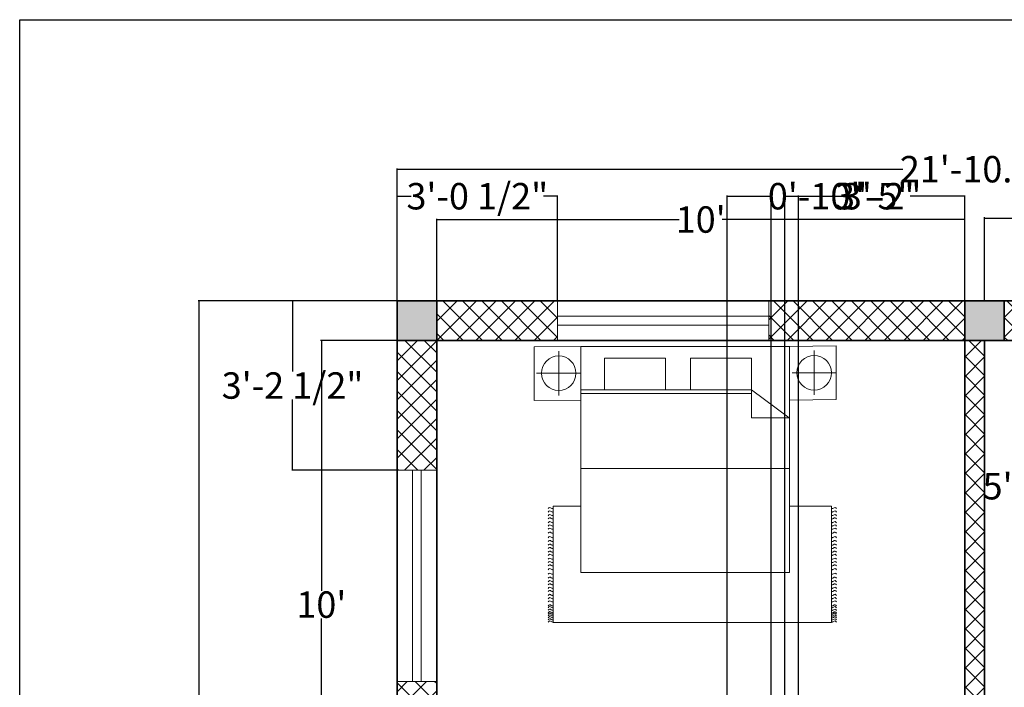
# Model space of a CAD drawing. Units: inches. Extents: x 958 to 1375, y 3152 to 3689.
# Tile 6 of 8: x 958 to 1182, y 3538 to 3689. Entities that reach past the tile are written whole.
import ezdxf

# ---------------------------------------------------------------- set-up
doc = ezdxf.new("R2010")
doc.units = ezdxf.units.IN
doc.header["$MEASUREMENT"] = 0
for name, color, linetype, lineweight in [('A-ANNO-DIMS', 2, 'Continuous', 18), ('A-ANNO-TTLB', 7, 'Continuous', 25), ('A-COLS', 7, 'Continuous', 35), ('A-FURN', 8, 'Continuous', 18), ('A-WALL', 7, 'Continuous', 35), ('windows', 140, 'Continuous', 18)]:
    doc.layers.add(name, color=color, linetype=linetype, lineweight=lineweight)
doc.layers.add('A-COLS-PATT', color=18, linetype='Continuous', lineweight=13, true_color=0x000000)
doc.layers.add('A-WALL-PATT', color=240, linetype='Continuous', lineweight=13, true_color=0xed1f24)
doc.styles.get("Standard").update_dxf_attribs({"font": 'arial.ttf'})
doc.dimstyles.get("Standard").update_dxf_attribs({"dimtxt": 6, "dimasz": 0.18, "dimexe": 0.18, "dimexo": 0.0625, "dimgap": 0.09, "dimtad": 0, "dimtih": 1, "dimtoh": 1, "dimdec": 1, "dimzin": 0, "dimdsep": 46, "dimlunit": 3, "dimtxsty": 'Standard', "dimcen": 0.09, "dimadec": 0, "dimazin": 0, "dimtfac": 1, "dimtdec": 1, "dimtofl": 0, "dimtmove": 0, "dimatfit": 3, "dimfxl": 1, "dimtolj": 1, "dimtzin": 0, "dimarcsym": 0})

# ---------------------------------------------------------------- blocks, each defined once
blk = doc.blocks.new('*D3')
at = {"layer": 'A-ANNO-DIMS', "color": 0, "lineweight": -2, "transparency": 16777216}
for p, q in [((1053.2, 3625.6), (1053.2, 3644.17)), ((1053.38, 3643.99), (1108.3, 3643.99)), ((1173.02, 3643.99), (1118.1, 3643.99)), ((1173.2, 3625.6), (1173.2, 3644.17))]:
    blk.add_line(p, q, dxfattribs=at)
at = {"layer": 'A-ANNO-DIMS', "color": 0, "transparency": 16777216}
for points in [[(1053.38, 3644.02), (1053.38, 3643.96), (1053.2, 3643.99)], [(1173.02, 3644.02), (1173.02, 3643.96), (1173.2, 3643.99)]]:
    blk.add_solid(points, dxfattribs=at)
at = {"layer": 'Defpoints', "color": 0, "transparency": 16777216}
for p in [(1173.2, 3643.99), (1053.2, 3625.53), (1173.2, 3625.53)]:
    blk.add_point(p, dxfattribs=at)
at = {"layer": 'A-ANNO-DIMS', "color": 0, "transparency": 16777216, "insert": (1113.2, 3643.99), "char_height": 6, "attachment_point": 5}
blk.add_mtext("\\A1;10'", dxfattribs=at)
blk = doc.blocks.new('*D4')
at = {"layer": 'A-ANNO-DIMS', "color": 0, "lineweight": -2, "transparency": 16777216}
for p, q in [((1177.7, 3625.6), (1177.7, 3644.49)), ((1177.88, 3644.31), (1232.8, 3644.31)), ((1297.52, 3644.31), (1242.6, 3644.31)), ((1297.7, 3625.6), (1297.7, 3644.49))]:
    blk.add_line(p, q, dxfattribs=at)
at = {"layer": 'A-ANNO-DIMS', "color": 0, "transparency": 16777216}
for points in [[(1177.88, 3644.34), (1177.88, 3644.28), (1177.7, 3644.31)], [(1297.52, 3644.34), (1297.52, 3644.28), (1297.7, 3644.31)]]:
    blk.add_solid(points, dxfattribs=at)
at = {"layer": 'Defpoints', "color": 0, "transparency": 16777216}
for p in [(1297.7, 3644.31), (1177.7, 3625.53), (1297.7, 3625.53)]:
    blk.add_point(p, dxfattribs=at)
at = {"layer": 'A-ANNO-DIMS', "color": 0, "transparency": 16777216, "insert": (1237.7, 3644.31), "char_height": 6, "attachment_point": 5}
blk.add_mtext("\\A1;10'", dxfattribs=at)
blk = doc.blocks.new('*D11')
at = {"layer": 'A-ANNO-DIMS', "color": 0, "lineweight": -2, "transparency": 16777216}
for p, q in [((1044.2, 3625.6), (1044.2, 3655.6)), ((1044.38, 3655.42), (1159.17, 3655.42)), ((1306.52, 3655.42), (1191.72, 3655.42)), ((1306.7, 3625.6), (1306.7, 3655.6))]:
    blk.add_line(p, q, dxfattribs=at)
at = {"layer": 'A-ANNO-DIMS', "color": 0, "transparency": 16777216}
for points in [[(1044.38, 3655.45), (1044.38, 3655.39), (1044.2, 3655.42)], [(1306.52, 3655.45), (1306.52, 3655.39), (1306.7, 3655.42)]]:
    blk.add_solid(points, dxfattribs=at)
at = {"layer": 'Defpoints', "color": 0, "transparency": 16777216}
for p in [(1306.7, 3655.42), (1044.2, 3625.53), (1306.7, 3625.53)]:
    blk.add_point(p, dxfattribs=at)
at = {"layer": 'A-ANNO-DIMS', "color": 0, "transparency": 16777216, "insert": (1175.45, 3655.42), "char_height": 6, "attachment_point": 5}
blk.add_mtext('\\A1;21\'-10.5"', dxfattribs=at)
blk = doc.blocks.new('*D12')
at = {"layer": 'A-ANNO-DIMS', "color": 0, "lineweight": -2, "transparency": 16777216}
for p, q in [((1044.13, 3616.53), (1026.81, 3616.53)), ((1026.99, 3616.35), (1026.99, 3559.69)), ((1026.99, 3496.71), (1026.99, 3553.38)), ((1044.13, 3496.53), (1026.81, 3496.53))]:
    blk.add_line(p, q, dxfattribs=at)
at = {"layer": 'A-ANNO-DIMS', "color": 0, "transparency": 16777216}
for points in [[(1026.96, 3616.35), (1027.02, 3616.35), (1026.99, 3616.53)], [(1026.96, 3496.71), (1027.02, 3496.71), (1026.99, 3496.53)]]:
    blk.add_solid(points, dxfattribs=at)
at = {"layer": 'Defpoints', "color": 0, "transparency": 16777216}
for p in [(1044.2, 3616.53), (1026.99, 3496.53), (1044.2, 3496.53)]:
    blk.add_point(p, dxfattribs=at)
at = {"layer": 'A-ANNO-DIMS', "color": 0, "transparency": 16777216, "insert": (1026.99, 3556.53), "char_height": 6, "attachment_point": 5}
blk.add_mtext("\\A1;10'", dxfattribs=at)
blk = doc.blocks.new('*D15')
at = {"layer": 'A-ANNO-DIMS', "color": 0, "lineweight": -2, "transparency": 16777216}
for p, q in [((1044.13, 3625.53), (998.97, 3625.53)), ((999.15, 3625.35), (999.15, 3444.94)), ((999.15, 3258.21), (999.15, 3438.63)), ((1044.13, 3258.03), (998.97, 3258.03))]:
    blk.add_line(p, q, dxfattribs=at)
at = {"layer": 'A-ANNO-DIMS', "color": 0, "transparency": 16777216}
for points in [[(999.12, 3625.35), (999.18, 3625.35), (999.15, 3625.53)], [(999.12, 3258.21), (999.18, 3258.21), (999.15, 3258.03)]]:
    blk.add_solid(points, dxfattribs=at)
at = {"layer": 'Defpoints', "color": 0, "transparency": 16777216}
for p in [(1044.2, 3625.53), (999.15, 3258.03), (1044.2, 3258.03)]:
    blk.add_point(p, dxfattribs=at)
at = {"layer": 'A-ANNO-DIMS', "color": 0, "transparency": 16777216, "insert": (999.15, 3441.78), "char_height": 6, "attachment_point": 5}
blk.add_mtext('\\A1;30\'-7.5"', dxfattribs=at)
blk = doc.blocks.new('BED-DOUBLE')
for p, q in [((5.6, 61.62), (5.6, 51.56)), ((63.65, 61.72), (63.65, 51.66)), ((10.63, 56.59), (0.57, 56.59)), ((68.68, 56.69), (58.62, 56.69)), ((49.39, 52.82), (10.63, 52.82)), ((49.44, 52), (10.63, 52)), ((49.39, 52.82), (58, 46.47)), ((49.44, 52.82), (49.44, 46.47)), ((49.44, 46.47), (58, 46.47)), ((58.05, 34.96), (10.63, 34.96)), ((4.36, 0), (4.36, 26.37)), ((4.36, 26.37), (10.65, 26.37)), ((58.05, 26.37), (67.59, 26.37)), ((67.59, 26.37), (67.59, 0)), ((67.59, 0), (4.36, 0))]:
    blk.add_line(p, q)
for points in [[(0, 50.39), (10.63, 50.5), (10.63, 62.68), (0, 62.58)], [(58.05, 62.68), (58.05, 11.37), (10.63, 11.37), (10.63, 62.68)], [(58.05, 50.5), (68.68, 50.6), (68.68, 62.78), (58.05, 62.68)], [(29.88, 59.98), (29.88, 52.82), (15.98, 52.82), (15.98, 59.98)], [(49.44, 59.98), (49.44, 52.82), (35.55, 52.82), (35.55, 59.98)]]:
    blk.add_lwpolyline(points, close=True)
for centre in [(5.6, 56.59), (63.65, 56.69)]:
    blk.add_circle(centre, 3.92)
for points, knots in [([(3.23, 25.84), (3.32, 25.96), (3.52, 26.2), (3.86, 25.96), (4.14, 25.78), (4.29, 25.89), (4.36, 25.94)], [0, 0, 0, 0, 0.400747, 0.791423, 1.067667, 1.29709, 1.29709, 1.29709, 1.29709]), ([(3.23, 25.06), (3.32, 25.18), (3.52, 25.42), (3.86, 25.18), (4.14, 25.01), (4.29, 25.11), (4.36, 25.16)], [0, 0, 0, 0, 0.400747, 0.791423, 1.067667, 1.29709, 1.29709, 1.29709, 1.29709]), ([(68.71, 25.84), (68.61, 25.96), (68.42, 26.2), (68.08, 25.96), (67.8, 25.78), (67.65, 25.89), (67.58, 25.94)], [0, 0, 0, 0, 0.400747, 0.791423, 1.067667, 1.29709, 1.29709, 1.29709, 1.29709]), ([(68.71, 25.06), (68.61, 25.18), (68.42, 25.42), (68.08, 25.18), (67.8, 25.01), (67.65, 25.11), (67.58, 25.16)], [0, 0, 0, 0, 0.400747, 0.791423, 1.067667, 1.29709, 1.29709, 1.29709, 1.29709]), ([(3.23, 24.24), (3.32, 24.36), (3.52, 24.6), (3.86, 24.36), (4.14, 24.19), (4.29, 24.3), (4.36, 24.34)], [0, 0, 0, 0, 0.400747, 0.791423, 1.067667, 1.29709, 1.29709, 1.29709, 1.29709]), ([(3.23, 23.51), (3.32, 23.63), (3.52, 23.87), (3.86, 23.63), (4.14, 23.46), (4.29, 23.57), (4.36, 23.62)], [0, 0, 0, 0, 0.400747, 0.791423, 1.067667, 1.29709, 1.29709, 1.29709, 1.29709]), ([(3.23, 22.63), (3.32, 22.75), (3.52, 22.99), (3.86, 22.75), (4.14, 22.58), (4.29, 22.69), (4.36, 22.73)], [0, 0, 0, 0, 0.400747, 0.791423, 1.067667, 1.29709, 1.29709, 1.29709, 1.29709]), ([(68.71, 24.24), (68.61, 24.36), (68.42, 24.6), (68.08, 24.36), (67.8, 24.19), (67.65, 24.3), (67.58, 24.34)], [0, 0, 0, 0, 0.400747, 0.791423, 1.067667, 1.29709, 1.29709, 1.29709, 1.29709]), ([(68.71, 23.51), (68.61, 23.63), (68.42, 23.87), (68.08, 23.63), (67.8, 23.46), (67.65, 23.57), (67.58, 23.62)], [0, 0, 0, 0, 0.400747, 0.791423, 1.067667, 1.29709, 1.29709, 1.29709, 1.29709]), ([(68.71, 22.63), (68.61, 22.75), (68.42, 22.99), (68.08, 22.75), (67.8, 22.58), (67.65, 22.69), (67.58, 22.73)], [0, 0, 0, 0, 0.400747, 0.791423, 1.067667, 1.29709, 1.29709, 1.29709, 1.29709]), ([(3.23, 21.88), (3.32, 22), (3.52, 22.24), (3.86, 22), (4.14, 21.83), (4.29, 21.93), (4.36, 21.98)], [0, 0, 0, 0, 0.400747, 0.791423, 1.067667, 1.29709, 1.29709, 1.29709, 1.29709]), ([(3.23, 21.15), (3.32, 21.27), (3.52, 21.51), (3.86, 21.27), (4.14, 21.1), (4.29, 21.21), (4.36, 21.25)], [0, 0, 0, 0, 0.400747, 0.791423, 1.067667, 1.29709, 1.29709, 1.29709, 1.29709]), ([(3.23, 20.27), (3.32, 20.39), (3.52, 20.63), (3.86, 20.39), (4.14, 20.22), (4.29, 20.32), (4.36, 20.37)], [0, 0, 0, 0, 0.400747, 0.791423, 1.067667, 1.29709, 1.29709, 1.29709, 1.29709]), ([(68.71, 21.88), (68.61, 22), (68.42, 22.24), (68.08, 22), (67.8, 21.83), (67.65, 21.93), (67.58, 21.98)], [0, 0, 0, 0, 0.400747, 0.791423, 1.067667, 1.29709, 1.29709, 1.29709, 1.29709]), ([(68.71, 21.15), (68.61, 21.27), (68.42, 21.51), (68.08, 21.27), (67.8, 21.1), (67.65, 21.21), (67.58, 21.25)], [0, 0, 0, 0, 0.400747, 0.791423, 1.067667, 1.29709, 1.29709, 1.29709, 1.29709]), ([(68.71, 20.27), (68.61, 20.39), (68.42, 20.63), (68.08, 20.39), (67.8, 20.22), (67.65, 20.32), (67.58, 20.37)], [0, 0, 0, 0, 0.400747, 0.791423, 1.067667, 1.29709, 1.29709, 1.29709, 1.29709]), ([(3.23, 19.23), (3.32, 19.35), (3.52, 19.59), (3.86, 19.35), (4.14, 19.18), (4.29, 19.29), (4.36, 19.33)], [0, 0, 0, 0, 0.400747, 0.791423, 1.067667, 1.29709, 1.29709, 1.29709, 1.29709]), ([(3.23, 18.35), (3.32, 18.47), (3.52, 18.71), (3.86, 18.47), (4.14, 18.3), (4.29, 18.4), (4.36, 18.45)], [0, 0, 0, 0, 0.400747, 0.791423, 1.067667, 1.29709, 1.29709, 1.29709, 1.29709]), ([(68.71, 19.23), (68.61, 19.35), (68.42, 19.59), (68.08, 19.35), (67.8, 19.18), (67.65, 19.29), (67.58, 19.33)], [0, 0, 0, 0, 0.400747, 0.791423, 1.067667, 1.29709, 1.29709, 1.29709, 1.29709]), ([(68.71, 18.35), (68.61, 18.47), (68.42, 18.71), (68.08, 18.47), (67.8, 18.3), (67.65, 18.4), (67.58, 18.45)], [0, 0, 0, 0, 0.400747, 0.791423, 1.067667, 1.29709, 1.29709, 1.29709, 1.29709]), ([(3.23, 17.53), (3.32, 17.65), (3.52, 17.89), (3.86, 17.65), (4.14, 17.48), (4.29, 17.59), (4.36, 17.64)], [0, 0, 0, 0, 0.400747, 0.791423, 1.067667, 1.29709, 1.29709, 1.29709, 1.29709]), ([(3.23, 16.76), (3.32, 16.88), (3.52, 17.12), (3.86, 16.88), (4.14, 16.71), (4.29, 16.81), (4.36, 16.86)], [0, 0, 0, 0, 0.400747, 0.791423, 1.067667, 1.29709, 1.29709, 1.29709, 1.29709]), ([(3.23, 15.94), (3.32, 16.06), (3.52, 16.3), (3.86, 16.06), (4.14, 15.89), (4.29, 16), (4.36, 16.04)], [0, 0, 0, 0, 0.400747, 0.791423, 1.067667, 1.29709, 1.29709, 1.29709, 1.29709]), ([(68.71, 17.53), (68.61, 17.65), (68.42, 17.89), (68.08, 17.65), (67.8, 17.48), (67.65, 17.59), (67.58, 17.64)], [0, 0, 0, 0, 0.400747, 0.791423, 1.067667, 1.29709, 1.29709, 1.29709, 1.29709]), ([(68.71, 16.76), (68.61, 16.88), (68.42, 17.12), (68.08, 16.88), (67.8, 16.71), (67.65, 16.81), (67.58, 16.86)], [0, 0, 0, 0, 0.400747, 0.791423, 1.067667, 1.29709, 1.29709, 1.29709, 1.29709]), ([(68.71, 15.94), (68.61, 16.06), (68.42, 16.3), (68.08, 16.06), (67.8, 15.89), (67.65, 16), (67.58, 16.04)], [0, 0, 0, 0, 0.400747, 0.791423, 1.067667, 1.29709, 1.29709, 1.29709, 1.29709]), ([(3.23, 15.21), (3.32, 15.33), (3.52, 15.57), (3.86, 15.33), (4.14, 15.16), (4.29, 15.27), (4.36, 15.32)], [0, 0, 0, 0, 0.400747, 0.791423, 1.067667, 1.29709, 1.29709, 1.29709, 1.29709]), ([(3.23, 14.33), (3.32, 14.45), (3.52, 14.69), (3.86, 14.45), (4.14, 14.28), (4.29, 14.39), (4.36, 14.43)], [0, 0, 0, 0, 0.400747, 0.791423, 1.067667, 1.29709, 1.29709, 1.29709, 1.29709]), ([(3.23, 13.58), (3.32, 13.7), (3.52, 13.94), (3.86, 13.7), (4.14, 13.53), (4.29, 13.63), (4.36, 13.68)], [0, 0, 0, 0, 0.400747, 0.791423, 1.067667, 1.29709, 1.29709, 1.29709, 1.29709]), ([(68.71, 15.21), (68.61, 15.33), (68.42, 15.57), (68.08, 15.33), (67.8, 15.16), (67.65, 15.27), (67.58, 15.32)], [0, 0, 0, 0, 0.400747, 0.791423, 1.067667, 1.29709, 1.29709, 1.29709, 1.29709]), ([(68.71, 14.33), (68.61, 14.45), (68.42, 14.69), (68.08, 14.45), (67.8, 14.28), (67.65, 14.39), (67.58, 14.43)], [0, 0, 0, 0, 0.400747, 0.791423, 1.067667, 1.29709, 1.29709, 1.29709, 1.29709]), ([(68.71, 13.58), (68.61, 13.7), (68.42, 13.94), (68.08, 13.7), (67.8, 13.53), (67.65, 13.63), (67.58, 13.68)], [0, 0, 0, 0, 0.400747, 0.791423, 1.067667, 1.29709, 1.29709, 1.29709, 1.29709]), ([(3.23, 12.85), (3.32, 12.97), (3.52, 13.21), (3.86, 12.97), (4.14, 12.8), (4.29, 12.9), (4.36, 12.95)], [0, 0, 0, 0, 0.400747, 0.791423, 1.067667, 1.29709, 1.29709, 1.29709, 1.29709]), ([(3.23, 11.97), (3.32, 12.09), (3.52, 12.33), (3.86, 12.09), (4.14, 11.92), (4.29, 12.02), (4.36, 12.07)], [0, 0, 0, 0, 0.400747, 0.791423, 1.067667, 1.29709, 1.29709, 1.29709, 1.29709]), ([(3.23, 10.93), (3.32, 11.05), (3.52, 11.29), (3.86, 11.05), (4.14, 10.88), (4.29, 10.99), (4.36, 11.03)], [0, 0, 0, 0, 0.400747, 0.791423, 1.067667, 1.29709, 1.29709, 1.29709, 1.29709]), ([(68.71, 12.85), (68.61, 12.97), (68.42, 13.21), (68.08, 12.97), (67.8, 12.8), (67.65, 12.9), (67.58, 12.95)], [0, 0, 0, 0, 0.400747, 0.791423, 1.067667, 1.29709, 1.29709, 1.29709, 1.29709]), ([(68.71, 11.97), (68.61, 12.09), (68.42, 12.33), (68.08, 12.09), (67.8, 11.92), (67.65, 12.02), (67.58, 12.07)], [0, 0, 0, 0, 0.400747, 0.791423, 1.067667, 1.29709, 1.29709, 1.29709, 1.29709]), ([(68.71, 10.93), (68.61, 11.05), (68.42, 11.29), (68.08, 11.05), (67.8, 10.88), (67.65, 10.99), (67.58, 11.03)], [0, 0, 0, 0, 0.400747, 0.791423, 1.067667, 1.29709, 1.29709, 1.29709, 1.29709]), ([(3.23, 10.05), (3.32, 10.17), (3.52, 10.41), (3.86, 10.17), (4.14, 10), (4.29, 10.1), (4.36, 10.15)], [0, 0, 0, 0, 0.400747, 0.791423, 1.067667, 1.29709, 1.29709, 1.29709, 1.29709]), ([(3.23, 9.23), (3.32, 9.35), (3.52, 9.59), (3.86, 9.35), (4.14, 9.18), (4.29, 9.29), (4.36, 9.34)], [0, 0, 0, 0, 0.400747, 0.791423, 1.067667, 1.29709, 1.29709, 1.29709, 1.29709]), ([(68.71, 10.05), (68.61, 10.17), (68.42, 10.41), (68.08, 10.17), (67.8, 10), (67.65, 10.1), (67.58, 10.15)], [0, 0, 0, 0, 0.400747, 0.791423, 1.067667, 1.29709, 1.29709, 1.29709, 1.29709]), ([(68.71, 9.23), (68.61, 9.35), (68.42, 9.59), (68.08, 9.35), (67.8, 9.18), (67.65, 9.29), (67.58, 9.34)], [0, 0, 0, 0, 0.400747, 0.791423, 1.067667, 1.29709, 1.29709, 1.29709, 1.29709]), ([(3.23, 8.54), (3.32, 8.66), (3.52, 8.9), (3.86, 8.66), (4.14, 8.49), (4.29, 8.6), (4.36, 8.65)], [0, 0, 0, 0, 0.400747, 0.791423, 1.067667, 1.29709, 1.29709, 1.29709, 1.29709]), ([(3.23, 7.73), (3.32, 7.85), (3.52, 8.09), (3.86, 7.85), (4.14, 7.68), (4.29, 7.78), (4.36, 7.83)], [0, 0, 0, 0, 0.400747, 0.791423, 1.067667, 1.29709, 1.29709, 1.29709, 1.29709]), ([(3.23, 7), (3.32, 7.12), (3.52, 7.36), (3.86, 7.12), (4.14, 6.95), (4.29, 7.05), (4.36, 7.1)], [0, 0, 0, 0, 0.400747, 0.791423, 1.067667, 1.29709, 1.29709, 1.29709, 1.29709]), ([(68.71, 8.54), (68.61, 8.66), (68.42, 8.9), (68.08, 8.66), (67.8, 8.49), (67.65, 8.6), (67.58, 8.65)], [0, 0, 0, 0, 0.400747, 0.791423, 1.067667, 1.29709, 1.29709, 1.29709, 1.29709]), ([(68.71, 7.73), (68.61, 7.85), (68.42, 8.09), (68.08, 7.85), (67.8, 7.68), (67.65, 7.78), (67.58, 7.83)], [0, 0, 0, 0, 0.400747, 0.791423, 1.067667, 1.29709, 1.29709, 1.29709, 1.29709]), ([(68.71, 7), (68.61, 7.12), (68.42, 7.36), (68.08, 7.12), (67.8, 6.95), (67.65, 7.05), (67.58, 7.1)], [0, 0, 0, 0, 0.400747, 0.791423, 1.067667, 1.29709, 1.29709, 1.29709, 1.29709]), ([(3.23, 6.12), (3.32, 6.24), (3.52, 6.48), (3.86, 6.24), (4.14, 6.07), (4.29, 6.17), (4.36, 6.22)], [0, 0, 0, 0, 0.400747, 0.791423, 1.067667, 1.29709, 1.29709, 1.29709, 1.29709]), ([(3.23, 5.37), (3.32, 5.49), (3.52, 5.73), (3.86, 5.49), (4.14, 5.31), (4.29, 5.42), (4.36, 5.47)], [0, 0, 0, 0, 0.400747, 0.791423, 1.067667, 1.29709, 1.29709, 1.29709, 1.29709]), ([(3.23, 4.64), (3.32, 4.76), (3.52, 5), (3.86, 4.76), (4.14, 4.59), (4.29, 4.69), (4.36, 4.74)], [0, 0, 0, 0, 0.400747, 0.791423, 1.067667, 1.29709, 1.29709, 1.29709, 1.29709]), ([(68.71, 6.12), (68.61, 6.24), (68.42, 6.48), (68.08, 6.24), (67.8, 6.07), (67.65, 6.17), (67.58, 6.22)], [0, 0, 0, 0, 0.400747, 0.791423, 1.067667, 1.29709, 1.29709, 1.29709, 1.29709]), ([(68.71, 5.37), (68.61, 5.49), (68.42, 5.73), (68.08, 5.49), (67.8, 5.31), (67.65, 5.42), (67.58, 5.47)], [0, 0, 0, 0, 0.400747, 0.791423, 1.067667, 1.29709, 1.29709, 1.29709, 1.29709]), ([(68.71, 4.64), (68.61, 4.76), (68.42, 5), (68.08, 4.76), (67.8, 4.59), (67.66, 4.69), (67.59, 4.73)], [0, 0, 0, 0, 0.400747, 0.791423, 1.067667, 1.283686, 1.283686, 1.283686, 1.283686]), ([(3.23, 3.75), (3.32, 3.88), (3.52, 4.12), (3.86, 3.88), (4.14, 3.7), (4.29, 3.81), (4.36, 3.86)], [0, 0, 0, 0, 0.400747, 0.791423, 1.067667, 1.29709, 1.29709, 1.29709, 1.29709]), ([(3.23, 3.33), (3.32, 3.45), (3.52, 3.7), (3.86, 3.45), (4.14, 3.27), (4.29, 3.38), (4.36, 3.43)], [0, 0, 0, 0, 0.407265, 0.802015, 1.07826, 1.307683, 1.307683, 1.307683, 1.307683]), ([(3.23, 2.76), (3.32, 2.88), (3.52, 3.12), (3.86, 2.88), (4.14, 2.71), (4.29, 2.81), (4.36, 2.86)], [0, 0, 0, 0, 0.400747, 0.791423, 1.067667, 1.29709, 1.29709, 1.29709, 1.29709]), ([(3.23, 2.19), (3.32, 2.31), (3.52, 2.55), (3.86, 2.31), (4.14, 2.13), (4.29, 2.24), (4.36, 2.29)], [0, 0, 0, 0, 0.400747, 0.791423, 1.067667, 1.29709, 1.29709, 1.29709, 1.29709]), ([(68.71, 3.75), (68.61, 3.88), (68.42, 4.12), (68.08, 3.88), (67.8, 3.7), (67.66, 3.81), (67.59, 3.85)], [0, 0, 0, 0, 0.400747, 0.791423, 1.067667, 1.283686, 1.283686, 1.283686, 1.283686]), ([(68.71, 3.33), (68.61, 3.45), (68.42, 3.69), (68.08, 3.45), (67.8, 3.28), (67.66, 3.38), (67.59, 3.42)], [0, 0, 0, 0, 0.402903, 0.794912, 1.071156, 1.287177, 1.287177, 1.287177, 1.287177]), ([(68.71, 2.73), (68.61, 2.85), (68.42, 3.09), (68.08, 2.85), (67.8, 2.68), (67.66, 2.78), (67.59, 2.83)], [0, 0, 0, 0, 0.400747, 0.791423, 1.067667, 1.283686, 1.283686, 1.283686, 1.283686]), ([(68.71, 2.16), (68.61, 2.28), (68.42, 2.52), (68.08, 2.28), (67.8, 2.11), (67.66, 2.21), (67.59, 2.25)], [0, 0, 0, 0, 0.400747, 0.791423, 1.067667, 1.283686, 1.283686, 1.283686, 1.283686]), ([(3.23, 1.88), (3.32, 2), (3.52, 2.24), (3.86, 2), (4.14, 1.82), (4.29, 1.93), (4.36, 1.98)], [0, 0, 0, 0, 0.400747, 0.791423, 1.067667, 1.29709, 1.29709, 1.29709, 1.29709]), ([(3.23, 1.46), (3.32, 1.58), (3.52, 1.82), (3.86, 1.58), (4.14, 1.41), (4.29, 1.51), (4.36, 1.56)], [0, 0, 0, 0, 0.400747, 0.791423, 1.067667, 1.29709, 1.29709, 1.29709, 1.29709]), ([(3.23, 1.06), (3.32, 1.18), (3.52, 1.42), (3.86, 1.18), (4.14, 1.01), (4.29, 1.11), (4.36, 1.16)], [0, 0, 0, 0, 0.400747, 0.791423, 1.067667, 1.29709, 1.29709, 1.29709, 1.29709]), ([(3.23, 0.57), (3.32, 0.7), (3.52, 0.94), (3.86, 0.7), (4.14, 0.52), (4.29, 0.63), (4.36, 0.68)], [0, 0, 0, 0, 0.400747, 0.791423, 1.067667, 1.29709, 1.29709, 1.29709, 1.29709]), ([(3.23, 0.07), (3.32, 0.19), (3.52, 0.43), (3.86, 0.19), (4.14, 0.02), (4.29, 0.13), (4.36, 0.18)], [0, 0, 0, 0, 0.400747, 0.791423, 1.067667, 1.29709, 1.29709, 1.29709, 1.29709]), ([(68.71, 1.43), (68.61, 1.55), (68.42, 1.79), (68.08, 1.55), (67.8, 1.38), (67.65, 1.48), (67.58, 1.53)], [0, 0, 0, 0, 0.400747, 0.791423, 1.067667, 1.29709, 1.29709, 1.29709, 1.29709]), ([(68.71, 1.03), (68.61, 1.15), (68.42, 1.39), (68.08, 1.15), (67.8, 0.98), (67.65, 1.09), (67.58, 1.13)], [0, 0, 0, 0, 0.400747, 0.791423, 1.067667, 1.29709, 1.29709, 1.29709, 1.29709]), ([(68.71, 0.55), (68.61, 0.67), (68.42, 0.91), (68.08, 0.67), (67.8, 0.5), (67.65, 0.6), (67.58, 0.65)], [0, 0, 0, 0, 0.400747, 0.791423, 1.067667, 1.29709, 1.29709, 1.29709, 1.29709]), ([(68.71, 0.07), (68.61, 0.19), (68.42, 0.43), (68.08, 0.19), (67.8, 0.02), (67.65, 0.13), (67.58, 0.18)], [0, 0, 0, 0, 0.400747, 0.791423, 1.067667, 1.29709, 1.29709, 1.29709, 1.29709]), ([(68.71, 1.85), (68.61, 1.97), (68.42, 2.21), (68.08, 1.97), (67.8, 1.8), (67.66, 1.9), (67.59, 1.94)], [0, 0, 0, 0, 0.400747, 0.791423, 1.067667, 1.283686, 1.283686, 1.283686, 1.283686])]:
    blk.add_open_spline(points, degree=3, knots=knots)
blk = doc.blocks.new('WIN-48')
for p, q in [((48, 9), (0, 9)), ((48, 5.5), (0, 5.5)), ((0, 3.5), (48, 3.5)), ((0, 0), (48, 0))]:
    blk.add_line(p, q)
blk = doc.blocks.new('*D27')
at = {"layer": 'A-ANNO-DIMS', "color": 0, "lineweight": -2, "transparency": 16777216}
for p, q in [((1205.81, 3614.81), (1195.39, 3614.81)), ((1195.57, 3614.63), (1195.57, 3586.57)), ((1195.57, 3552.21), (1195.57, 3580.26)), ((1205.81, 3552.03), (1195.39, 3552.03))]:
    blk.add_line(p, q, dxfattribs=at)
at = {"layer": 'A-ANNO-DIMS', "color": 0, "transparency": 16777216}
for points in [[(1195.54, 3614.63), (1195.6, 3614.63), (1195.57, 3614.81)], [(1195.54, 3552.21), (1195.6, 3552.21), (1195.57, 3552.03)]]:
    blk.add_solid(points, dxfattribs=at)
at = {"layer": 'Defpoints', "color": 0, "transparency": 16777216}
for p in [(1195.57, 3614.81), (1205.88, 3614.81), (1205.88, 3552.03)]:
    blk.add_point(p, dxfattribs=at)
at = {"layer": 'A-ANNO-DIMS', "color": 0, "transparency": 16777216, "insert": (1195.57, 3583.42), "char_height": 6, "attachment_point": 5}
blk.add_mtext('\\A1;5\'-3" TYP.', dxfattribs=at)
blk = doc.blocks.new('*D43')
at = {"layer": 'A-ANNO-DIMS', "color": 0, "lineweight": -2, "transparency": 16777216}
for p, q in [((1119.2, 3303.1), (1119.2, 3649.46)), ((1119.38, 3649.28), (1129.02, 3649.28)), ((1129.2, 3303.1), (1129.2, 3649.46)), ((1129.2, 3649.28), (1129.38, 3649.28))]:
    blk.add_line(p, q, dxfattribs=at)
at = {"layer": 'A-ANNO-DIMS', "color": 0, "transparency": 16777216}
for points in [[(1119.38, 3649.31), (1119.38, 3649.25), (1119.2, 3649.28)], [(1129.02, 3649.31), (1129.02, 3649.25), (1129.2, 3649.28)]]:
    blk.add_solid(points, dxfattribs=at)
at = {"layer": 'Defpoints', "color": 0, "transparency": 16777216}
for p in [(1129.2, 3649.28), (1119.2, 3303.03), (1129.2, 3303.03)]:
    blk.add_point(p, dxfattribs=at)
at = {"layer": 'A-ANNO-DIMS', "color": 0, "transparency": 16777216, "insert": (1139.77, 3649.28), "char_height": 6, "attachment_point": 5}
blk.add_mtext('\\A1;0\'-10"', dxfattribs=at)
blk = doc.blocks.new('*D44')
at = {"layer": 'A-ANNO-DIMS', "color": 0, "lineweight": -2, "transparency": 16777216}
for p, q in [((1132.32, 3267.1), (1132.32, 3649.46)), ((1132.5, 3649.28), (1144.69, 3649.28)), ((1173.02, 3649.28), (1160.82, 3649.28)), ((1173.2, 3267.1), (1173.2, 3649.46))]:
    blk.add_line(p, q, dxfattribs=at)
at = {"layer": 'A-ANNO-DIMS', "color": 0, "transparency": 16777216}
for points in [[(1132.5, 3649.31), (1132.5, 3649.25), (1132.32, 3649.28)], [(1173.02, 3649.31), (1173.02, 3649.25), (1173.2, 3649.28)]]:
    blk.add_solid(points, dxfattribs=at)
at = {"layer": 'Defpoints', "color": 0, "transparency": 16777216}
for p in [(1173.2, 3649.28), (1132.32, 3267.03), (1173.2, 3267.03)]:
    blk.add_point(p, dxfattribs=at)
at = {"layer": 'A-ANNO-DIMS', "color": 0, "transparency": 16777216, "insert": (1152.76, 3649.28), "char_height": 6, "attachment_point": 5}
blk.add_mtext('\\A1;3\'-5"', dxfattribs=at)
blk = doc.blocks.new('*D46')
at = {"layer": 'A-ANNO-DIMS', "color": 0, "lineweight": -2, "transparency": 16777216}
for p, q in [((1135.44, 3496.6), (1135.44, 3649.46)), ((1135.62, 3649.28), (1146.25, 3649.28)), ((1173.02, 3649.28), (1162.38, 3649.28)), ((1173.2, 3492.1), (1173.2, 3649.46))]:
    blk.add_line(p, q, dxfattribs=at)
at = {"layer": 'A-ANNO-DIMS', "color": 0, "transparency": 16777216}
for points in [[(1135.62, 3649.31), (1135.62, 3649.25), (1135.44, 3649.28)], [(1173.02, 3649.31), (1173.02, 3649.25), (1173.2, 3649.28)]]:
    blk.add_solid(points, dxfattribs=at)
at = {"layer": 'Defpoints', "color": 0, "transparency": 16777216}
for p in [(1173.2, 3649.28), (1135.44, 3496.53), (1173.2, 3492.03)]:
    blk.add_point(p, dxfattribs=at)
at = {"layer": 'A-ANNO-DIMS', "color": 0, "transparency": 16777216, "insert": (1154.32, 3649.28), "char_height": 6, "attachment_point": 5}
blk.add_mtext('\\A1;3\'-2"', dxfattribs=at)
blk = doc.blocks.new('*D50')
at = {"layer": 'A-ANNO-DIMS', "color": 0, "lineweight": -2, "transparency": 16777216}
for p, q in [((1044.2, 3625.6), (1044.2, 3649.46)), ((1044.38, 3649.28), (1047.39, 3649.28)), ((1080.5, 3649.28), (1077.49, 3649.28)), ((1080.68, 3625.6), (1080.68, 3649.46))]:
    blk.add_line(p, q, dxfattribs=at)
at = {"layer": 'A-ANNO-DIMS', "color": 0, "transparency": 16777216}
for points in [[(1044.38, 3649.31), (1044.38, 3649.25), (1044.2, 3649.28)], [(1080.5, 3649.31), (1080.5, 3649.25), (1080.68, 3649.28)]]:
    blk.add_solid(points, dxfattribs=at)
at = {"layer": 'Defpoints', "color": 0, "transparency": 16777216}
for p in [(1080.68, 3649.28), (1044.2, 3625.53), (1080.68, 3625.53)]:
    blk.add_point(p, dxfattribs=at)
at = {"layer": 'A-ANNO-DIMS', "color": 0, "transparency": 16777216, "insert": (1062.44, 3649.28), "char_height": 6, "attachment_point": 5}
blk.add_mtext('\\A1;3\'-0 1/2"', dxfattribs=at)
blk = doc.blocks.new('*D52')
at = {"layer": 'A-ANNO-DIMS', "color": 0, "lineweight": -2, "transparency": 16777216}
for p, q in [((1044.13, 3625.53), (1020.27, 3625.53)), ((1020.45, 3625.35), (1020.45, 3609.49)), ((1020.45, 3587.23), (1020.45, 3603.1)), ((1044.13, 3587.05), (1020.27, 3587.05))]:
    blk.add_line(p, q, dxfattribs=at)
at = {"layer": 'A-ANNO-DIMS', "color": 0, "transparency": 16777216}
for points in [[(1020.42, 3625.35), (1020.48, 3625.35), (1020.45, 3625.53)], [(1020.42, 3587.23), (1020.48, 3587.23), (1020.45, 3587.05)]]:
    blk.add_solid(points, dxfattribs=at)
at = {"layer": 'Defpoints', "color": 0, "transparency": 16777216}
for p in [(1020.45, 3625.53), (1044.2, 3625.53), (1044.2, 3587.05)]:
    blk.add_point(p, dxfattribs=at)
at = {"layer": 'A-ANNO-DIMS', "color": 0, "transparency": 16777216, "insert": (1020.45, 3606.29), "char_height": 6, "attachment_point": 5}
blk.add_mtext('\\A1;3\'-2 1/2"', dxfattribs=at)

msp = doc.modelspace()

# ---------------------------------------------------------------- hatches: boundary and pattern name
at = {"layer": 'A-COLS-PATT'}
h = msp.add_hatch(color=256, dxfattribs=at)
h.dxf.hatch_style = 1
h.paths.add_polyline_path([(1053.2, 3625.53), (1044.2, 3625.53), (1044.2, 3616.53), (1053.2, 3616.53)])
h.paths.add_polyline_path([(1182.2, 3625.53), (1173.2, 3625.53), (1173.2, 3616.53), (1182.2, 3616.53)])
h.paths.add_polyline_path([(1306.7, 3625.53), (1297.7, 3625.53), (1297.7, 3616.53), (1306.7, 3616.53)])
h.paths.add_polyline_path([(1306.7, 3501.03), (1297.7, 3501.03), (1297.7, 3492.03), (1306.7, 3492.03)])
h.paths.add_polyline_path([(1306.7, 3391.53), (1297.7, 3391.53), (1297.7, 3382.53), (1306.7, 3382.53)])
h.paths.add_polyline_path([(1306.7, 3267.03), (1297.7, 3267.03), (1297.7, 3258.03), (1306.7, 3258.03)])
h.paths.add_polyline_path([(1182.2, 3267.03), (1173.2, 3267.03), (1173.2, 3258.03), (1182.2, 3258.03)])
h.paths.add_polyline_path([(1053.2, 3267.03), (1044.2, 3267.03), (1044.2, 3258.03), (1053.2, 3258.03)])
h.paths.add_polyline_path([(1053.2, 3391.53), (1044.2, 3391.53), (1044.2, 3382.53), (1053.2, 3382.53)])
h.paths.add_polyline_path([(1053.2, 3501.03), (1044.2, 3501.03), (1044.2, 3492.03), (1053.2, 3492.03)])
h.paths.add_polyline_path([(1182.2, 3501.03), (1173.2, 3501.03), (1173.2, 3492.03), (1182.2, 3492.03)])
h.paths.add_polyline_path([(1182.2, 3391.53), (1173.2, 3391.53), (1173.2, 3382.53), (1182.2, 3382.53)])
at = {"layer": 'A-WALL-PATT'}
h = msp.add_hatch(dxfattribs=at)
h.set_pattern_fill('ANSI37', color=256, scale=25)
h.paths.add_polyline_path([(1080.68, 3625.53), (1053.2, 3625.53), (1053.2, 3616.53), (1080.68, 3616.53)])
h.paths.add_polyline_path([(1053.2, 3616.53), (1044.2, 3616.53), (1044.2, 3587.05), (1053.2, 3587.05)])
h.paths.add_polyline_path([(1173.2, 3625.53), (1128.68, 3625.53), (1128.68, 3616.53), (1173.2, 3616.53)])
h.paths.add_polyline_path([(1215.78, 3625.53), (1182.2, 3625.53), (1182.2, 3616.53), (1215.78, 3616.53)])
h.paths.add_polyline_path([(1297.7, 3625.53), (1263.78, 3625.53), (1263.78, 3616.53), (1297.7, 3616.53)])
h.paths.add_polyline_path([(1177.7, 3616.53), (1173.2, 3616.53), (1173.2, 3501.03), (1177.7, 3501.03)])
h.paths.add_polyline_path([(1053.2, 3539.05), (1044.2, 3539.05), (1044.2, 3501.03), (1053.2, 3501.03)])
h.paths.add_polyline_path([(1135.44, 3496.53), (1053.2, 3496.53), (1053.2, 3492.03), (1135.44, 3492.03)])
h.paths.add_polyline_path([(1306.7, 3616.53), (1297.7, 3616.53), (1297.7, 3586.38), (1306.7, 3586.38)])
h.paths.add_polyline_path([(1306.7, 3538.38), (1297.7, 3538.38), (1297.7, 3501.03), (1306.7, 3501.03)])
h.paths.add_polyline_path([(1297.7, 3496.53), (1216.84, 3496.53), (1216.84, 3492.03), (1297.7, 3492.03)])
h.paths.add_polyline_path([(1306.7, 3492.03), (1297.7, 3492.03), (1297.7, 3481.63), (1306.7, 3481.63)])
h.paths.add_polyline_path([(1306.7, 3457.63), (1297.7, 3457.63), (1297.7, 3444.03), (1225.7, 3444.03), (1225.7, 3462.51), (1221.2, 3462.51), (1221.2, 3391.53), (1182.2, 3391.53), (1182.2, 3387.03), (1225.7, 3387.03), (1225.7, 3439.53), (1297.7, 3439.53), (1297.7, 3428.57), (1306.7, 3428.57)])
h.paths.add_polyline_path([(1306.7, 3404.57), (1297.7, 3404.57), (1297.7, 3391.53), (1306.7, 3391.53)], flags=17)
h.paths.add_polyline_path([(1297.7, 3391.53), (1253.12, 3391.53), (1253.12, 3387.03), (1297.7, 3387.03)], flags=17)
h.paths.add_polyline_path([(1306.7, 3382.53), (1297.7, 3382.53), (1297.7, 3354.01), (1306.7, 3354.01)])
h.paths.add_polyline_path([(1306.7, 3306.01), (1297.7, 3306.01), (1297.7, 3267.03), (1306.7, 3267.03)])
h.paths.add_polyline_path([(1297.7, 3267.03), (1254.05, 3267.03), (1254.05, 3258.03), (1297.7, 3258.03)])
h.paths.add_polyline_path([(1177.7, 3347.74), (1173.2, 3347.74), (1173.2, 3267.03), (1177.7, 3267.03)])
h.paths.add_polyline_path([(1206.05, 3267.03), (1182.2, 3267.03), (1182.2, 3258.03), (1206.05, 3258.03)])
h.paths.add_polyline_path([(1053.2, 3308.96), (1044.2, 3308.96), (1044.2, 3267.03), (1053.2, 3267.03)])
h.paths.add_polyline_path([(1053.2, 3382.53), (1044.2, 3382.53), (1044.2, 3356.96), (1053.2, 3356.96)])
h.paths.add_polyline_path([(1053.2, 3420.58), (1044.2, 3420.58), (1044.2, 3391.53), (1053.2, 3391.53)])
h.paths.add_polyline_path([(1053.2, 3492.03), (1044.2, 3492.03), (1044.2, 3468.58), (1053.2, 3468.58)])

# ---------------------------------------------------------------- linework, layer by layer
at = {"layer": 'A-ANNO-TTLB'}
msp.add_lwpolyline([(958.44, 3689.37), (1374.91, 3689.37), (1374.91, 3152.28), (958.44, 3152.28)], close=True, dxfattribs=at)
at = {"layer": 'A-COLS'}
for p, q in [((1173.2, 3625.53), (1182.2, 3625.53)), ((1182.2, 3625.53), (1182.2, 3616.53)), ((1182.2, 3616.53), (1173.2, 3616.53))]:
    msp.add_line(p, q, dxfattribs=at)
at = {"layer": 'A-WALL'}
for p, q in [((1044.2, 3625.53), (1306.7, 3625.53)), ((1044.2, 3625.53), (1044.2, 3258.03)), ((1053.2, 3625.53), (1053.2, 3258.03)), ((1173.2, 3625.53), (1173.2, 3492.03)), ((1173.2, 3625.53), (1173.2, 3492.03)), ((1044.2, 3616.53), (1306.7, 3616.53)), ((1177.7, 3616.53), (1177.7, 3501.03)), ((1177.7, 3616.53), (1177.7, 3501.03))]:
    msp.add_line(p, q, dxfattribs=at)
at = {"layer": 'windows'}
for p, q in [((1080.68, 3625.53), (1080.68, 3616.53)), ((1128.68, 3616.53), (1128.68, 3625.53)), ((1044.2, 3587.05), (1053.2, 3587.05)), ((1053.2, 3539.05), (1044.2, 3539.05))]:
    msp.add_line(p, q, dxfattribs=at)

# ---------------------------------------------------------------- block references
at = {"layer": 'A-FURN'}
msp.add_blockref('BED-DOUBLE', (1075.34, 3552.49), dxfattribs=at)
at = {"layer": 'windows'}
msp.add_blockref('WIN-48', (1080.68, 3616.53), dxfattribs=at)
at = {"layer": 'windows', "rotation": 90}
msp.add_blockref('WIN-48', (1053.2, 3539.05), dxfattribs=at)

# ---------------------------------------------------------------- dimensions: what is measured, and where the dimension line sits
at = {"layer": 'A-ANNO-DIMS'}
for base, p1, p2, override, picture, middle in [((1306.7, 3655.42), (1044.2, 3625.53), (1306.7, 3625.53), {"dimclrd": 0, "dimclre": 0, "dimclrt": 0}, '*D11', (1175.45, 3655.42)), ((1080.68, 3649.28), (1044.2, 3625.53), (1080.68, 3625.53), {"dimdec": 1, "dimlfac": 1, "dimrnd": 0, "dimzin": 1, "dimdsep": 46, "dimlunit": 4, "dimfrac": 2}, '*D50', (1062.44, 3649.28)), ((1129.2, 3649.28), (1119.2, 3303.03), (1129.2, 3303.03), {"dimdec": 1, "dimlfac": 1, "dimrnd": 0, "dimzin": 1, "dimdsep": 46, "dimlunit": 4, "dimfrac": 2}, '*D43', (1139.77, 3649.28)), ((1173.2, 3649.28), (1132.32, 3267.03), (1173.2, 3267.03), {"dimdec": 1, "dimlfac": 1, "dimrnd": 0, "dimzin": 1, "dimdsep": 46, "dimlunit": 4, "dimfrac": 2}, '*D44', (1152.76, 3649.28)), ((1173.2, 3649.28), (1135.44, 3496.53), (1173.2, 3492.03), {"dimdec": 1, "dimlfac": 1, "dimrnd": 0, "dimzin": 1, "dimdsep": 46, "dimlunit": 4, "dimfrac": 2}, '*D46', (1154.32, 3649.28)), ((1173.2, 3643.99), (1053.2, 3625.53), (1173.2, 3625.53), {"dimclrd": 0, "dimclre": 0, "dimclrt": 0}, '*D3', (1113.2, 3643.99)), ((1297.7, 3644.31), (1177.7, 3625.53), (1297.7, 3625.53), {"dimclrd": 0, "dimclre": 0, "dimclrt": 0}, '*D4', (1237.7, 3644.31))]:
    dim = msp.add_linear_dim(base=base, p1=p1, p2=p2, dimstyle='Standard', override=override, dxfattribs=at)
    dim.commit()
    dim.dimension.update_dxf_attribs({"geometry": picture, "text_midpoint": middle})
for base, p1, p2, override, picture, middle in [((999.15, 3258.03), (1044.2, 3625.53), (1044.2, 3258.03), {"dimclrd": 0, "dimclre": 0, "dimclrt": 0}, '*D15', (999.15, 3441.78)), ((1020.45, 3625.53), (1044.2, 3587.05), (1044.2, 3625.53), {"dimdec": 1, "dimlfac": 1, "dimrnd": 0, "dimzin": 1, "dimdsep": 46, "dimlunit": 4, "dimfrac": 2}, '*D52', (1020.45, 3606.29)), ((1026.99, 3496.53), (1044.2, 3616.53), (1044.2, 3496.53), {"dimclrd": 0, "dimclre": 0, "dimclrt": 0}, '*D12', (1026.99, 3556.53))]:
    dim = msp.add_linear_dim(base=base, p1=p1, p2=p2, angle=90, dimstyle='Standard', override=override, dxfattribs=at)
    dim.commit()
    dim.dimension.update_dxf_attribs({"geometry": picture, "text_midpoint": middle})
dim = msp.add_linear_dim(base=(1195.57, 3614.81), p1=(1205.88, 3552.03), p2=(1205.88, 3614.81), angle=90, text='<> TYP.', dimstyle='Standard', override={"dimdec": 1, "dimlfac": 1, "dimrnd": 0, "dimzin": 1, "dimdsep": 46, "dimlunit": 4, "dimfrac": 2}, dxfattribs=at)
dim.commit()
dim.dimension.update_dxf_attribs({"geometry": '*D27', "text_midpoint": (1195.57, 3583.42)})

doc.saveas('drawing.dxf')
